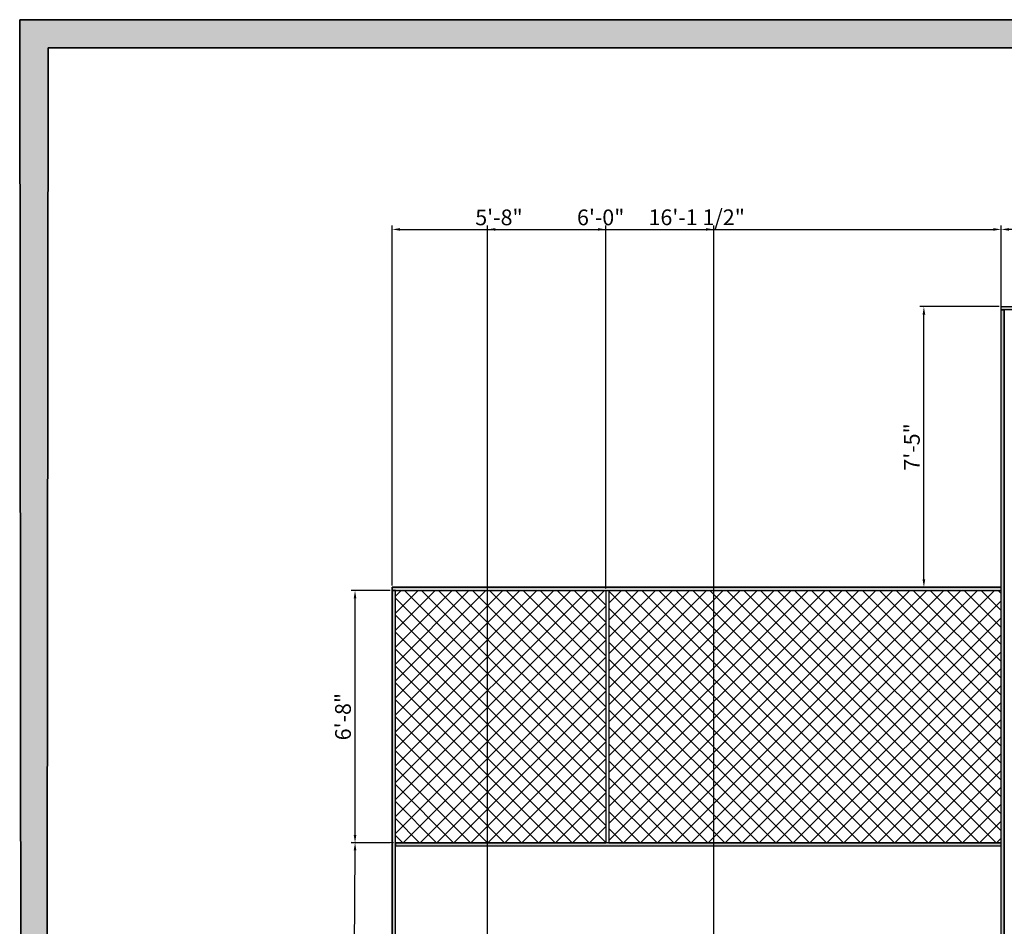
# Model space of a CAD drawing. Units: inches. Extents: x 1804 to 3296, y 909 to 2477.
# Tile 27 of 31: x 1804 to 2117, y 2188 to 2477. Entities that reach past the tile are written whole.
import ezdxf

# ---------------------------------------------------------------- set-up
doc = ezdxf.new("R2010")
doc.units = ezdxf.units.IN
for name, color, linetype, lineweight in [('A-ANNO-DIMS', 2, 'Continuous', 18), ('A-ANNO-TTLB', 156, 'Continuous', 35), ('A-ELEV-PATT', 85, 'Continuous', 13), ('ELE', 210, 'Continuous', 30)]:
    doc.layers.add(name, color=color, linetype=linetype, lineweight=lineweight)
doc.styles.get("Standard").update_dxf_attribs({"font": 'arial.ttf'})
doc.dimstyles.new('ISO-25', dxfattribs={"dimtxt": 5, "dimasz": 2.5, "dimexe": 1.25, "dimexo": 0.625, "dimtad": 1, "dimdec": 0, "dimlunit": 4, "dimtxsty": 'Standard', "dimcen": 2.5, "dimadec": 0, "dimazin": 0, "dimtfac": 1, "dimtdec": 0, "dimtmove": 0, "dimatfit": 3, "dimfxl": 1, "dimarcsym": 0})

# ---------------------------------------------------------------- blocks, each defined once
blk = doc.blocks.new('*D29')
at = {"layer": 'A-ANNO-DIMS', "color": 0, "lineweight": -2, "transparency": 16777216}
for p, q in [((1922.54, 2214.87), (1909.11, 2214.95)), ((1909.37, 2052.89), (1910.34, 2212.44)), ((1921.54, 2050.32), (1908.11, 2050.4))]:
    blk.add_line(p, q, dxfattribs=at)
at = {"layer": 'A-ANNO-DIMS', "color": 0, "lineweight": 100, "transparency": 16777216}
for points in [[(1909.93, 2212.44), (1910.76, 2212.44), (1910.36, 2214.94)], [(1908.96, 2052.89), (1909.79, 2052.89), (1909.36, 2050.39)]]:
    blk.add_solid(points, dxfattribs=at)
at = {"layer": 'Defpoints', "color": 0, "lineweight": 100, "transparency": 16777216}
for p in [(1910.36, 2214.94), (1923.17, 2214.86), (1922.17, 2050.31)]:
    blk.add_point(p, dxfattribs=at)
at = {"layer": 'A-ANNO-DIMS', "color": 0, "transparency": 16777216, "insert": (1906.68, 2132.68), "char_height": 5, "attachment_point": 5, "rotation": 89.6518}
blk.add_mtext('13\'-9"', dxfattribs=at)
blk = doc.blocks.new('*D30')
at = {"layer": 'A-ANNO-DIMS', "color": 0, "lineweight": -2, "transparency": 16777216}
for p, q in [((1921.54, 2295.08), (1909.1, 2295.08)), ((1910.35, 2217.36), (1910.35, 2292.58)), ((1921.54, 2214.86), (1909.1, 2214.86))]:
    blk.add_line(p, q, dxfattribs=at)
at = {"layer": 'A-ANNO-DIMS', "color": 0, "lineweight": 100, "transparency": 16777216}
for points in [[(1909.93, 2292.58), (1910.77, 2292.58), (1910.35, 2295.08)], [(1909.93, 2217.36), (1910.77, 2217.36), (1910.35, 2214.86)]]:
    blk.add_solid(points, dxfattribs=at)
at = {"layer": 'Defpoints', "color": 0, "lineweight": 100, "transparency": 16777216}
for p in [(1910.35, 2295.08), (1922.17, 2295.08), (1922.17, 2214.86)]:
    blk.add_point(p, dxfattribs=at)
at = {"layer": 'A-ANNO-DIMS', "color": 0, "transparency": 16777216, "insert": (1907.17, 2254.97), "char_height": 5, "attachment_point": 5, "rotation": 90}
blk.add_mtext('6\'-8"', dxfattribs=at)
blk = doc.blocks.new('*D31')
at = {"layer": 'A-ANNO-DIMS', "color": 0, "lineweight": -2, "transparency": 16777216}
for p, q in [((2115.04, 2385.31), (2089.87, 2385.31)), ((2091.12, 2298.58), (2091.12, 2382.81)), ((2115.04, 2296.08), (2089.87, 2296.08))]:
    blk.add_line(p, q, dxfattribs=at)
at = {"layer": 'A-ANNO-DIMS', "color": 0, "lineweight": 100, "transparency": 16777216}
for points in [[(2090.7, 2382.81), (2091.54, 2382.81), (2091.12, 2385.31)], [(2090.7, 2298.58), (2091.54, 2298.58), (2091.12, 2296.08)]]:
    blk.add_solid(points, dxfattribs=at)
at = {"layer": 'Defpoints', "color": 0, "lineweight": 100, "transparency": 16777216}
for p in [(2091.12, 2385.31), (2115.67, 2385.31), (2115.67, 2296.08)]:
    blk.add_point(p, dxfattribs=at)
at = {"layer": 'A-ANNO-DIMS', "color": 0, "transparency": 16777216, "insert": (2087.95, 2340.7), "char_height": 5, "attachment_point": 5, "rotation": 90}
blk.add_mtext('7\'-5"', dxfattribs=at)
blk = doc.blocks.new('*D76')
at = {"layer": 'A-ANNO-DIMS', "color": 0, "lineweight": -2, "transparency": 16777216}
for p, q in [((1922.17, 2296.71), (1922.17, 2411.11)), ((1924.67, 2409.86), (2113.17, 2409.86)), ((2115.67, 2296.71), (2115.67, 2411.11))]:
    blk.add_line(p, q, dxfattribs=at)
at = {"layer": 'A-ANNO-DIMS', "color": 0, "lineweight": 100, "transparency": 16777216}
for points in [[(1924.67, 2410.28), (1924.67, 2409.44), (1922.17, 2409.86)], [(2113.17, 2410.28), (2113.17, 2409.44), (2115.67, 2409.86)]]:
    blk.add_solid(points, dxfattribs=at)
at = {"layer": 'Defpoints', "color": 0, "lineweight": 100, "transparency": 16777216}
for p in [(2115.67, 2409.86), (1922.17, 2296.08), (2115.67, 2296.08)]:
    blk.add_point(p, dxfattribs=at)
at = {"layer": 'A-ANNO-DIMS', "color": 0, "transparency": 16777216, "insert": (2018.92, 2413.07), "char_height": 5, "attachment_point": 5}
blk.add_mtext('16\'-1 1/2"', dxfattribs=at)
blk = doc.blocks.new('*D77')
at = {"layer": 'A-ANNO-DIMS', "color": 0, "lineweight": -2, "transparency": 16777216}
for p, q in [((1922.17, 2296.71), (1922.17, 2411.11)), ((1924.67, 2409.86), (1987.52, 2409.86)), ((1990.02, 2295.71), (1990.02, 2411.11))]:
    blk.add_line(p, q, dxfattribs=at)
at = {"layer": 'A-ANNO-DIMS', "color": 0, "lineweight": 100, "transparency": 16777216}
for points in [[(1924.67, 2410.28), (1924.67, 2409.44), (1922.17, 2409.86)], [(1987.52, 2410.28), (1987.52, 2409.44), (1990.02, 2409.86)]]:
    blk.add_solid(points, dxfattribs=at)
at = {"layer": 'Defpoints', "color": 0, "lineweight": 100, "transparency": 16777216}
for p in [(1990.02, 2409.86), (1922.17, 2296.08), (1990.02, 2295.08)]:
    blk.add_point(p, dxfattribs=at)
at = {"layer": 'A-ANNO-DIMS', "color": 0, "transparency": 16777216, "insert": (1956.09, 2413.04), "char_height": 5, "attachment_point": 5}
blk.add_mtext('5\'-8"', dxfattribs=at)
blk = doc.blocks.new('*D78')
at = {"layer": 'A-ANNO-DIMS', "color": 0, "lineweight": -2, "transparency": 16777216}
for p, q in [((1952.44, 2175.25), (1952.44, 2411.11)), ((1954.94, 2409.86), (2021.88, 2409.86)), ((2024.38, 2175.25), (2024.38, 2411.11))]:
    blk.add_line(p, q, dxfattribs=at)
at = {"layer": 'A-ANNO-DIMS', "color": 0, "lineweight": 100, "transparency": 16777216}
for points in [[(1954.94, 2410.28), (1954.94, 2409.44), (1952.44, 2409.86)], [(2021.88, 2410.28), (2021.88, 2409.44), (2024.38, 2409.86)]]:
    blk.add_solid(points, dxfattribs=at)
at = {"layer": 'Defpoints', "color": 0, "lineweight": 100, "transparency": 16777216}
for p in [(2024.38, 2409.86), (1952.44, 2174.63), (2024.38, 2174.63)]:
    blk.add_point(p, dxfattribs=at)
at = {"layer": 'A-ANNO-DIMS', "color": 0, "transparency": 16777216, "insert": (1988.41, 2413.04), "char_height": 5, "attachment_point": 5}
blk.add_mtext('6\'-0"', dxfattribs=at)
blk = doc.blocks.new('*D86')
at = {"layer": 'A-ANNO-DIMS', "color": 0, "lineweight": -2, "transparency": 16777216}
for p, q in [((2115.67, 2385.93), (2115.67, 2411.11)), ((2177.43, 2409.86), (2118.17, 2409.86)), ((2179.93, 2354.6), (2179.93, 2411.11))]:
    blk.add_line(p, q, dxfattribs=at)
at = {"layer": 'A-ANNO-DIMS', "color": 0, "lineweight": 100, "transparency": 16777216}
for points in [[(2118.17, 2410.28), (2118.17, 2409.44), (2115.67, 2409.86)], [(2177.43, 2410.28), (2177.43, 2409.44), (2179.93, 2409.86)]]:
    blk.add_solid(points, dxfattribs=at)
at = {"layer": 'Defpoints', "color": 0, "lineweight": 100, "transparency": 16777216}
for p in [(2115.67, 2409.86), (2115.67, 2385.31), (2179.93, 2353.97)]:
    blk.add_point(p, dxfattribs=at)
at = {"layer": 'A-ANNO-DIMS', "color": 0, "transparency": 16777216, "insert": (2147.8, 2413.07), "char_height": 5, "attachment_point": 5}
blk.add_mtext('5\'-4 1/2"', dxfattribs=at)

msp = doc.modelspace()

# ---------------------------------------------------------------- hatches: boundary and pattern name
at = {"layer": 'A-ANNO-TTLB'}
h = msp.add_hatch(color=256, dxfattribs=at)
h.dxf.hatch_style = 1
h.paths.add_polyline_path([(3294.53, 2476.54), (1803.79, 2476.54), (1805.43, 909.47), (3296.17, 909.47)])
h.paths.add_polyline_path([(1811, 914.33), (1812.79, 2467.54), (3285.53, 2467.54), (3283.74, 914.33)], flags=16)
h.paths.add_polyline_path([(1925.58, 1062.77), (1925.58, 1138.07), (1925.58, 1539.88), (1925.58, 1793.38), (1925.58, 1830.04), (2325.54, 1830.04), (2325.54, 1793.38), (2325.54, 1586.42), (2325.54, 1138.07), (2325.54, 1062.77)], flags=0)
h.paths.add_polyline_path([(1997.22, 1029.4), (2008.85, 1037.96), (2008.85, 1020.84)], flags=0)
h.paths.add_polyline_path([(1934.58, 1138.07), (1934.58, 1147.07), (2078.77, 1147.07), (2078.77, 1138.07), (2060.94, 1138.07)], flags=0)
h.paths.add_polyline_path([(1944.35, 1138.07), (1944.35, 1147.07), (2056.05, 1147.07), (2056.05, 1138.07)], flags=0)
h.paths.add_polyline_path([(2222.24, 1037.96), (2233.87, 1029.4), (2222.24, 1020.84)], flags=0)
h.paths.add_polyline_path([(2061.94, 1139.07), (2061.94, 1146.07), (2077.77, 1146.07), (2077.77, 1139.07)], flags=0)
h.paths.add_polyline_path([(2149.58, 1138.07), (2149.58, 1269.44), (2158.58, 1269.44), (2158.58, 1326.69), (2149.58, 1326.69), (2149.58, 1340.94), (2139.6, 1340.94), (2139.6, 1434.25), (2149.58, 1434.25), (2149.58, 1447.36), (2158.58, 1447.36), (2158.58, 1423.87), (2158.58, 1408.06), (2198.46, 1408.06), (2198.46, 1412.56), (2282.65, 1412.56), (2282.65, 1465.94), (2316.54, 1465.94), (2316.54, 1590.92), (2192.86, 1590.92), (2192.86, 1595.3), (2291.17, 1595.3), (2291.17, 1590.92), (2316.54, 1590.92), (2316.54, 1784.38), (2300.24, 1784.38), (2300.24, 1757.47), (2268, 1757.47), (2268, 1681.04), (2180.87, 1681.04), (2180.87, 1757.47), (2148.63, 1757.47), (2148.63, 1784.38), (2119.08, 1784.38), (2119.08, 1585.58), (2114.58, 1585.58), (2114.58, 1784.38), (2064.11, 1784.38), (2046.28, 1784.38), (2046.28, 1760.38), (1958.58, 1760.38), (1958.58, 1664.38), (1934.58, 1664.38), (1934.58, 1784.38), (1934.58, 1793.38), (2046.28, 1793.38), (2064.11, 1793.38), (2119.08, 1793.38), (2230.78, 1793.38), (2230.78, 1784.38), (2268, 1784.38), (2300.24, 1784.38), (2316.54, 1784.38), (2316.54, 1590.92), (2316.54, 1373.73), (2316.54, 1138.07)], flags=0)
h.paths.add_polyline_path([(2209.19, 1166.63), (2209.19, 1175.63), (2158.58, 1175.63), (2209.19, 1223.63), (2209.19, 1231.63), (2183.88, 1231.63), (2183.88, 1301.66), (2242.59, 1301.66), (2242.59, 1326.69), (2316.54, 1326.69), (2272.59, 1271.63), (2272.59, 1223.63), (2316.54, 1175.63), (2272.59, 1175.63), (2272.59, 1166.63)], flags=0)
h.paths.add_polyline_path([(1947.77, 1345.22), (1947.77, 1457.48), (1991.2, 1457.48), (1991.2, 1451.7), (1991.2, 1352.18), (1991.2, 1345.22)], flags=0)
h.paths.add_polyline_path([(2209.19, 1271.63), (2262.59, 1271.63), (2262.59, 1311.85), (2272.59, 1301.66), (2272.59, 1271.63), (2269.92, 1269.63), (2270.59, 1269.63), (2270.59, 1225.63), (2211.19, 1225.63), (2211.19, 1269.63), (2211.86, 1269.63)], flags=0)
h.paths.add_polyline_path([(2000.34, 1378.21), (2000.34, 1429.71), (2025.22, 1429.71), (2025.22, 1378.21)], flags=0)
h.paths.add_polyline_path([(2001.34, 1379.21), (2001.34, 1428.71), (2024.22, 1428.71), (2024.22, 1379.21)], flags=0)
h.paths.add_polyline_path([(2012.34, 1390.21), (2012.34, 1417.71), (2013.22, 1417.71), (2013.22, 1390.21)], flags=0)
h.paths.add_polyline_path([(2237.56, 1331.19), (2237.56, 1340.18), (2238.62, 1340.18), (2238.62, 1386.84), (2241.04, 1386.84), (2242.06, 1386.84), (2242.06, 1408.06), (2316.54, 1331.19)], flags=0)
h.paths.add_polyline_path([(1953.73, 1464.35), (1953.73, 1498.59), (1981.74, 1498.59), (1981.74, 1464.35)], flags=0)
h.paths.add_polyline_path([(1987.63, 1462.08), (1987.63, 1500.95), (2104.07, 1500.95), (2104.07, 1462.08), (2099.27, 1462.08), (1993.6, 1462.08)], flags=0)
h.paths.add_polyline_path([(1956.06, 1481.47, -1), (1979.41, 1481.47, -1)], flags=0)
edge = h.paths.add_edge_path(flags=0)
edge.add_ellipse((2299.53, 1438.37), major_axis=(0.31, 21.36), ratio=0.670333, start_angle=0, end_angle=360)
h.paths.add_polyline_path([(2297.39, 1438.37, -1), (2301.67, 1438.37, -1)], flags=0)
h.paths.add_polyline_path([(2591.54, 1163.23), (2591.54, 1179.38), (2591.54, 1379.68), (2591.54, 1395.84), (2734.5, 1395.84), (2734.5, 1379.68), (2734.5, 1179.38), (2734.5, 1163.23)], flags=0)
h.paths.add_polyline_path([(2592.54, 1164.23), (2592.54, 1166.23), (2733.5, 1166.23), (2733.5, 1164.23)], flags=0)
h.paths.add_polyline_path([(2592.54, 1180.38), (2592.54, 1378.68), (2733.5, 1378.68), (2733.5, 1180.38)], flags=0)
h.paths.add_polyline_path([(2593.54, 1181.38), (2593.54, 1377.68), (2732.5, 1377.68), (2732.5, 1181.38)], flags=0)
h.paths.add_polyline_path([(2594.54, 1182.38), (2594.54, 1376.68), (2731.5, 1376.68), (2731.5, 1182.38)], flags=0)
h.paths.add_polyline_path([(1936.95, 1697.46), (1936.95, 1736.46), (1955.41, 1736.46), (1955.41, 1697.46)], flags=0)
h.paths.add_polyline_path([(1938.48, 1718.36), (1938.48, 1734.92), (1953.65, 1734.92), (1953.65, 1718.36)], flags=0)
h.paths.add_polyline_path([(1944.75, 1726.64, -1), (1947.37, 1726.64, -1)], flags=0)
h.paths.add_polyline_path([(2592.54, 1394.84), (2733.5, 1394.84), (2733.5, 1392.84), (2592.54, 1392.84)], flags=0)
h.paths.add_polyline_path([(1976.61, 1762.5), (1976.61, 1781.44), (2012.79, 1781.44), (2012.79, 1762.5)], flags=0)
h.paths.add_polyline_path([(1979.57, 1771.97, -1), (1991.39, 1771.97, -1)], flags=0)
h.paths.add_polyline_path([(1995.36, 1771.97, -1), (2007.18, 1771.97, -1)], flags=0)
h.paths.add_polyline_path([(2251.51, 1744.53), (2268, 1730.05), (2251.51, 1730.05)], flags=0)
h.paths.add_polyline_path([(2047.28, 1785.38), (2047.28, 1792.38), (2063.11, 1792.38), (2063.11, 1785.38)], flags=0)
h.paths.add_polyline_path([(2155.08, 1770.92, -1), (2174.42, 1770.92, -1)], flags=0)
h.paths.add_polyline_path([(2188.59, 1758.27), (2188.59, 1772.81), (2222.3, 1772.81), (2222.3, 1758.27)], flags=0)
h.paths.add_polyline_path([(2223.97, 1758.27), (2223.97, 1772.81), (2257.68, 1772.81), (2257.68, 1758.27)], flags=0)
h.paths.add_polyline_path([(2274.45, 1770.92, -1), (2293.8, 1770.92, -1)], flags=0)
h.paths.add_polyline_path([(2591.54, 1582.09), (2591.54, 1782.39), (2734.5, 1782.39), (2734.5, 1582.09)], flags=0)
h.paths.add_polyline_path([(2592.54, 1583.09), (2592.54, 1781.39), (2733.5, 1781.39), (2733.5, 1583.09)], flags=0)
h.paths.add_polyline_path([(2593.54, 1584.09), (2593.54, 1780.39), (2732.5, 1780.39), (2732.5, 1584.09)], flags=0)
h.paths.add_polyline_path([(2594.54, 1585.09), (2594.54, 1779.39), (2731.5, 1779.39), (2731.5, 1585.09)], flags=0)
h.paths.add_polyline_path([(1922.17, 1978.79), (1922.17, 2295.08), (1922.17, 2296.08), (2115.67, 2296.08), (2115.67, 2384.31), (2115.67, 2385.31), (2322.12, 2385.31), (2323.12, 2385.31), (2323.12, 1979.79), (2323.12, 1978.79), (1923.17, 1978.79)], flags=0)
h.paths.add_polyline_path([(1922.17, 1978.79), (1922.17, 2051.31), (1922.17, 2214.86), (1922.17, 2296.08), (2115.67, 2296.08), (2115.67, 2385.31), (2323.12, 2385.31), (2323.12, 2280.42), (2323.12, 1978.79), (2115.67, 1978.79)], flags=0)
h.paths.add_polyline_path([(1923.17, 1979.79), (1923.17, 2050.31), (2115.67, 2050.31), (2115.67, 2051.31), (1923.17, 2051.31), (1923.17, 2213.86), (1923.17, 2214.86), (1923.17, 2295.08), (1990.02, 2295.08), (1990.02, 2214.86), (1991.02, 2214.86), (1991.02, 2295.08), (2115.67, 2295.08), (2115.67, 1979.79), (2116.67, 1979.79), (2116.67, 2304.18), (2116.67, 2384.31), (2322.12, 2384.31), (2322.12, 2280.42), (2322.12, 1979.79), (2115.67, 1979.79)], flags=0)
h.paths.add_polyline_path([(2972.46, 1192.5), (2972.46, 1196.92), (2995.47, 1196.92), (2995.47, 1255.47), (2995.09, 1255.47), (2987.42, 1249.39), (2980.08, 1255.47), (2978.05, 1255.47), (2978.05, 1257.24), (2995.47, 1257.24), (2995.47, 1261.58), (3015.37, 1261.58), (3015.37, 1333.28), (3015.37, 1414.4), (3032.82, 1414.4), (3032.82, 1333.28), (3032.82, 1261.58), (3052.66, 1261.58), (3052.66, 1255.47), (3079.86, 1255.47), (3078.72, 1254.57), (3081.47, 1252.29), (3078.56, 1249.99), (3075.81, 1252.26), (3072.57, 1249.69), (3070.36, 1251.52), (3067.67, 1249.39), (3060.34, 1255.47), (3052.66, 1255.47), (3052.66, 1196.92), (3054.58, 1196.92), (3074, 1196.92), (3074, 1192.5), (3052.66, 1192.5), (2995.47, 1192.5)], flags=0)
h.paths.add_polyline_path([(2490.75, 1979.27), (2490.75, 1980.27), (2596.87, 1980.27), (2596.87, 2051.8), (2596.87, 2052.8), (2596.87, 2216.35), (2596.87, 2297.57), (2717.32, 2297.57), (2710.57, 2305.62), (2724.07, 2305.62), (2717.32, 2297.57), (2782.37, 2297.57), (2782.37, 2395.8), (3006.82, 2395.8), (3006.82, 1981.27), (3093.73, 1981.27), (3093.73, 1980.27), (3047.51, 1980.27), (3046.37, 1979.37), (3049.11, 1977.1), (3046.2, 1974.79), (3043.46, 1977.07), (3040.21, 1974.49), (3038, 1976.32), (3035.32, 1974.2), (3027.98, 1980.27), (2871.83, 1980.27), (2871.83, 1981.27), (2791.37, 1981.27), (2791.37, 2050.8), (2597.87, 2050.8), (2597.87, 1980.27), (2597.87, 1979.27), (2546.27, 1979.27), (2545.12, 1978.37), (2547.87, 1976.1), (2544.96, 1973.79), (2542.22, 1976.07), (2538.97, 1973.49), (2536.76, 1975.32), (2534.07, 1973.2), (2526.74, 1979.27)], flags=0)
h.paths.add_polyline_path([(2597.87, 2051.8), (2606.87, 2051.8), (2606.87, 2258.39), (2597.87, 2258.39), (2597.87, 2296.57), (2606.87, 2296.57), (2606.87, 2262.39), (2782.37, 2262.39), (2782.37, 2296.57), (2790.37, 2296.57), (2790.37, 2262.39), (2791.37, 2262.39), (2791.37, 2305.67), (2791.37, 2385.8), (2996.82, 2385.8), (2996.82, 2339.85), (3006.82, 2339.85), (3006.82, 2250.12), (2997.82, 2250.12), (2997.82, 1981.27), (2996.82, 1981.27), (2872.83, 1981.27), (2872.83, 1991.8), (2871.83, 1991.8), (2871.83, 2050.8), (2790.37, 2050.8), (2597.87, 2050.8)], flags=0)
h.paths.add_polyline_path([(2179.93, 2153.92), (2179.93, 2353.97), (2259.98, 2353.97), (2259.98, 2153.92)], flags=0)
h.paths.add_polyline_path([(2180.93, 2154.92), (2180.93, 2352.97), (2258.98, 2352.97), (2258.98, 2154.92)], flags=0)
h.paths.add_polyline_path([(2960.87, 1608.49), (2960.87, 1753.62), (3070.9, 1753.62), (3070.9, 1608.49)], flags=0)
h.paths.add_polyline_path([(2961.87, 1609.49), (2961.87, 1752.62), (3069.9, 1752.62), (3069.9, 1609.49)], flags=0)
h.paths.add_polyline_path([(2962.87, 1610.49), (2962.87, 1751.62), (3068.9, 1751.62), (3068.9, 1610.49)], flags=0)
h.paths.add_polyline_path([(2963.87, 1611.49), (2963.87, 1750.62), (3067.9, 1750.62), (3067.9, 1611.49)], flags=0)
h.paths.add_polyline_path([(2782.37, 2051.8), (2782.37, 2216.32), (2791.37, 2216.32), (2791.37, 2051.8), (2872.83, 2051.8), (2872.83, 2068.56), (2884.67, 2068.56), (2884.67, 2085.33), (2896.51, 2085.33), (2896.51, 2102.09), (2908.36, 2102.09), (2908.36, 2118.85), (2920.2, 2118.85), (2920.2, 2135.62), (2932.05, 2135.62), (2932.05, 2145.3), (2925.08, 2145.3), (2925.08, 2203.2), (2996.82, 2203.2), (2996.82, 2145.3), (2953.82, 2145.3), (2872.83, 2051.8), (2790.37, 2051.8)], flags=0)
h.paths.add_polyline_path([(2717.32, 2238.65), (2710.57, 2246.7), (2724.07, 2246.7)], flags=0)
h.paths.add_polyline_path([(2003.09, 1122.79), (2017.16, 1122.79), (2017.16, 1138.74), (2003.09, 1138.74)], flags=8)
h.paths.add_polyline_path([(2174.76, 1792.72), (2188.83, 1792.72), (2188.83, 1808.66), (2174.76, 1808.66)], flags=8)
h.paths.add_polyline_path([(1987.95, 1792.51), (2002.02, 1792.51), (2002.02, 1808.45), (1987.95, 1808.45)], flags=8)
h.paths.add_polyline_path([(2148.79, 1289.26), (2160.46, 1289.26), (2160.46, 1305.2), (2148.79, 1305.2)], flags=8)
h.paths.add_polyline_path([(2115.36, 1133.57), (2127.04, 1133.57), (2127.04, 1149.51), (2115.36, 1149.51)], flags=8)
h.paths.add_polyline_path([(2237.58, 1421.48), (2249.25, 1421.48), (2249.25, 1437.43), (2237.58, 1437.43)], flags=8)
h.paths.add_polyline_path([(2134.99, 1584.32), (2146.66, 1584.32), (2146.66, 1600.26), (2134.99, 1600.26)], flags=8)
h.paths.add_polyline_path([(2101.95, 1557.31), (2113.62, 1557.31), (2113.62, 1573.25), (2101.95, 1573.25)], flags=8)
h.paths.add_polyline_path([(2937.85, 1156.77), (3120.41, 1156.77), (3120.41, 1185.72), (2937.85, 1185.72)], flags=8)
h.paths.add_polyline_path([(2980.71, 1786.71), (3050.06, 1786.71), (3050.06, 1802.66), (2980.71, 1802.66)], flags=8)
h.paths.add_polyline_path([(2869.28, 1661.96), (2938.62, 1661.96), (2938.62, 1690.8), (2869.28, 1690.8)], flags=8)
h.paths.add_polyline_path([(3092.27, 1674.86), (3161.62, 1674.86), (3161.62, 1690.8), (3092.27, 1690.8)], flags=8)
h.paths.add_polyline_path([(2980.71, 1674.86), (3050.06, 1674.86), (3050.06, 1690.8), (2980.71, 1690.8)], flags=8)
h.paths.add_polyline_path([(2649.07, 1678.23), (2674.53, 1678.23), (2674.53, 1714.76), (2649.07, 1714.76)], flags=8)
h.paths.add_polyline_path([(2530.84, 1981.63), (2549.13, 1981.63), (2549.13, 1997.57), (2530.84, 1997.57)], flags=8)
h.paths.add_polyline_path([(3031.29, 1981.77), (3049.58, 1981.77), (3049.58, 1997.71), (3031.29, 1997.71)], flags=8)
h.paths.add_polyline_path([(2715.38, 1911.9), (2851.54, 1911.9), (2851.54, 1940.85), (2715.38, 1940.85)], flags=8)
h.paths.add_polyline_path([(2015.23, 1927.36), (2205.42, 1927.36), (2205.42, 1956.3), (2015.23, 1956.3)], flags=8)
h.paths.add_polyline_path([(2671.84, 2057.84), (2702.75, 2057.84), (2702.75, 2073.79), (2671.84, 2073.79)], flags=8)
h.paths.add_polyline_path([(2678.5, 2316.52), (2765.26, 2316.52), (2765.26, 2332.46), (2678.5, 2332.46)], flags=8)
h.paths.add_polyline_path([(2678.48, 2271.96), (2736.41, 2271.96), (2736.41, 2287.9), (2678.48, 2287.9)], flags=8)
h.paths.add_polyline_path([(2019.2, 972.79), (2243.21, 972.79), (2243.21, 1001.74), (2019.2, 1001.74)], flags=8)
h.paths.add_polyline_path([(2097.06, 1021.56), (2132.16, 1021.56), (2132.16, 1037.51), (2097.06, 1037.51)], flags=8)
h.paths.add_polyline_path([(2182.47, 1360.48), (2207.35, 1360.48), (2207.35, 1376.42), (2182.47, 1376.42)], flags=8)
h.paths.add_polyline_path([(2261.12, 1361.77), (2295.01, 1361.77), (2295.01, 1377.71), (2261.12, 1377.71)], flags=8)
h.paths.add_polyline_path([(2245.75, 1511.51), (2278.44, 1511.51), (2278.44, 1527.46), (2245.75, 1527.46)], flags=8)
h.paths.add_polyline_path([(1991.16, 1296.29), (2060.51, 1296.29), (2060.51, 1312.23), (1991.16, 1312.23)], flags=8)
h.paths.add_polyline_path([(2187, 1651.35), (2246.71, 1651.35), (2246.71, 1667.29), (2187, 1667.29)], flags=8)
h.paths.add_polyline_path([(1976.49, 1684.81), (2068.63, 1684.81), (2068.63, 1700.76), (1976.49, 1700.76)], flags=8)
at = {"layer": 'A-ELEV-PATT'}
h = msp.add_hatch(color=256, dxfattribs=at)
h.dxf.hatch_style = 1
h.paths.add_polyline_path([(2322.12, 2385.31), (2115.67, 2385.31), (2115.67, 2384.31), (2322.12, 2384.31)])
h = msp.add_hatch(color=256, dxfattribs=at)
h.dxf.hatch_style = 1
h.paths.add_polyline_path([(2116.67, 2384.31), (2115.67, 2384.31), (2115.67, 1979.79), (2116.67, 1979.79)])
h = msp.add_hatch(color=256, dxfattribs=at)
h.dxf.hatch_style = 1
h.paths.add_polyline_path([(2115.67, 2296.08), (1922.17, 2296.08), (1922.17, 2295.08), (2115.67, 2295.08)])
h = msp.add_hatch(color=256, dxfattribs=at)
h.dxf.hatch_style = 1
h.paths.add_polyline_path([(1923.17, 2295.08), (1922.17, 2295.08), (1922.17, 1978.79), (1923.17, 1978.79)])
h = msp.add_hatch(dxfattribs=at)
h.set_pattern_fill('ANSI37', color=256, scale=1.2)
h.set_pattern_definition([(45, (-3.413, 129.5847), (-2.694077, 2.694077), []), (135, (-3.413, 129.5847), (-2.694077, -2.694077), [])])
h.paths.add_polyline_path([(1923.17, 2214.86), (1990.02, 2214.86), (1990.02, 2295.08), (1923.17, 2295.08)])
h.paths.add_polyline_path([(1991.02, 2214.86), (2115.67, 2214.86), (2115.67, 2295.08), (1991.02, 2295.08)])
h = msp.add_hatch(color=256, dxfattribs=at)
h.dxf.hatch_style = 1
h.paths.add_polyline_path([(2115.67, 2214.86), (1923.17, 2214.86), (1923.17, 2213.86), (2115.67, 2213.86)])

# ---------------------------------------------------------------- linework, layer by layer
at = {"layer": 'A-ANNO-TTLB'}
for points in [[(1803.79, 2476.54), (3294.53, 2476.54), (3296.17, 909.47), (1805.43, 909.47)], [(1812.79, 2467.54), (3285.53, 2467.54), (3283.74, 914.33), (1811, 914.33)]]:
    msp.add_lwpolyline(points, close=True, dxfattribs=at)
at = {"layer": 'ELE'}
for p, q in [((2115.67, 2296.08), (2115.67, 2385.31)), ((2115.67, 2385.31), (2323.12, 2385.31)), ((2116.67, 2296.08), (2116.67, 2384.31)), ((2115.67, 2296.08), (2115.67, 2304.18)), ((2116.67, 1979.79), (2116.67, 2304.18)), ((1922.17, 2214.86), (1922.17, 2296.08)), ((1922.17, 2296.08), (2115.67, 2296.08)), ((1923.17, 2295.08), (1990.02, 2295.08)), ((1923.17, 2214.86), (1923.17, 2295.08)), ((1990.02, 2295.08), (1990.02, 2214.86)), ((1991.02, 2295.08), (1991.02, 2214.86)), ((1991.02, 2295.08), (2115.67, 2295.08)), ((2115.67, 1979.79), (2115.67, 2295.08)), ((1922.17, 2051.31), (1922.17, 2214.86)), ((1923.17, 2214.86), (1990.02, 2214.86)), ((1923.17, 2213.86), (2115.67, 2213.86)), ((1923.17, 2051.31), (1923.17, 2213.86)), ((1991.02, 2214.86), (2115.67, 2214.86))]:
    msp.add_line(p, q, dxfattribs=at)
for points in [[(2115.67, 2385.31), (2322.12, 2385.31), (2322.12, 2384.31), (2115.67, 2384.31)], [(2115.67, 2384.31), (2116.67, 2384.31), (2116.67, 1979.79), (2115.67, 1979.79)], [(1922.17, 2295.08), (2115.67, 2295.08), (2115.67, 2296.08), (1922.17, 2296.08)], [(1922.17, 1978.79), (1923.17, 1978.79), (1923.17, 2295.08), (1922.17, 2295.08)], [(1923.17, 2213.86), (2115.67, 2213.86), (2115.67, 2214.86), (1923.17, 2214.86)]]:
    msp.add_lwpolyline(points, close=True, dxfattribs=at)

# ---------------------------------------------------------------- dimensions: what is measured, and where the dimension line sits
at = {"layer": 'A-ANNO-DIMS'}
for base, p1, p2, picture, middle in [((2115.67, 2409.86), (1922.17, 2296.08), (2115.67, 2296.08), '*D76', (2018.92, 2413.07)), ((2115.67, 2409.86), (2179.93, 2353.97), (2115.67, 2385.31), '*D86', (2147.8, 2413.07)), ((1990.0175, 2409.8598), (1922.1699, 2296.0845), (1990.0175, 2295.0845), '*D77', (1956.0937, 2413.0377)), ((2024.38, 2409.86), (1952.44, 2174.63), (2024.38, 2174.63), '*D78', (1988.41, 2413.04))]:
    dim = msp.add_linear_dim(base=base, p1=p1, p2=p2, dimstyle='ISO-25', override={"dimdec": 1, "dimlfac": 1, "dimrnd": 0, "dimzin": 1, "dimdsep": 46, "dimlunit": 4, "dimfrac": 2}, dxfattribs=at)
    dim.commit()
    dim.dimension.update_dxf_attribs({"geometry": picture, "text_midpoint": middle})
for base, p1, p2, picture, middle in [((2091.12, 2385.31), (2115.67, 2296.08), (2115.67, 2385.31), '*D31', (2087.95, 2340.7)), ((1910.35, 2295.08), (1922.17, 2214.86), (1922.17, 2295.08), '*D30', (1907.17, 2254.97))]:
    dim = msp.add_linear_dim(base=base, p1=p1, p2=p2, angle=90, dimstyle='ISO-25', override={"dimclrd": 0, "dimclre": 0, "dimclrt": 0}, dxfattribs=at)
    dim.commit()
    dim.dimension.update_dxf_attribs({"geometry": picture, "text_midpoint": middle})
dim = msp.add_aligned_dim(p1=(1922.17, 2050.31), p2=(1923.17, 2214.86), distance=12.81, dimstyle='ISO-25', override={"dimclrd": 0, "dimclre": 0, "dimclrt": 0}, dxfattribs=at)
dim.commit()
dim.dimension.update_dxf_attribs({"geometry": '*D29', "text_midpoint": (1906.68, 2132.68)})

doc.saveas('drawing.dxf')
